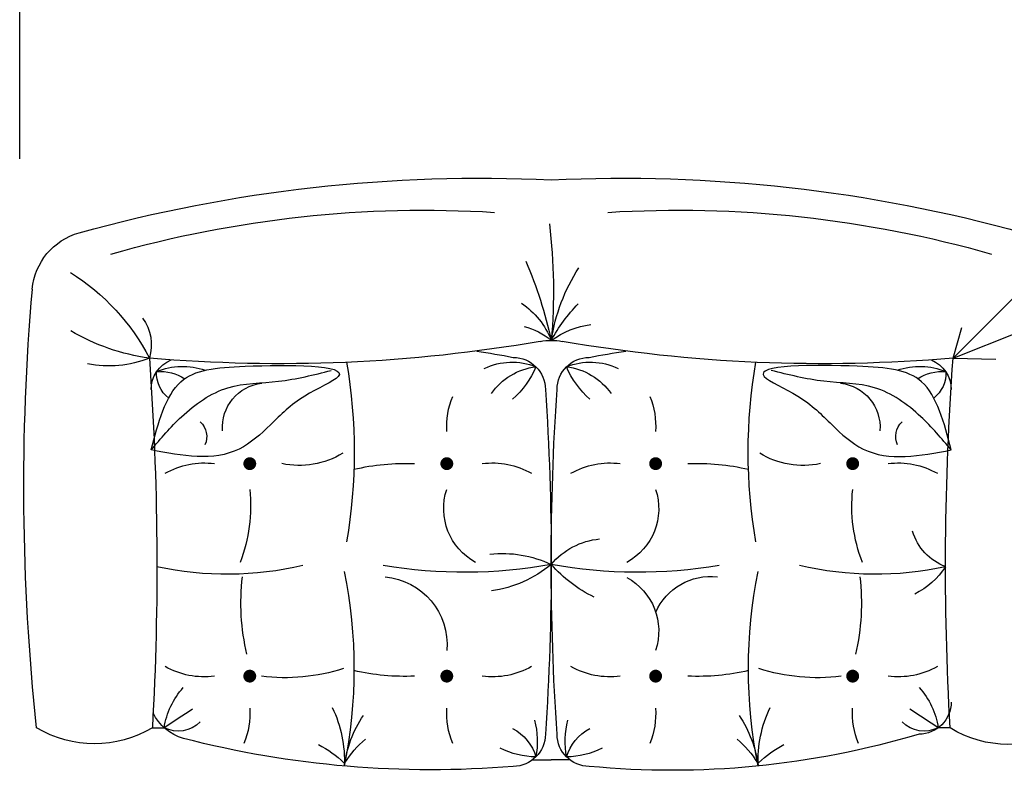
# Model space of a CAD drawing. Units: inches. Extents: x 3592 to 4861, y 1650 to 2243.
# Tile 9 of 30: x 4173 to 4219, y 1968 to 2003. Entities that reach past the tile are written whole.
import ezdxf

# ---------------------------------------------------------------- set-up
doc = ezdxf.new("R2010")
doc.units = ezdxf.units.IN
doc.layers.add('A-ANNO-DIMS', color=2, linetype='Continuous', lineweight=13)
doc.layers.add('A-FURN', color=9, linetype='Continuous', lineweight=13)
doc.layers.add('RA-AP-01$0$FURN', color=3, linetype='Continuous')
doc.styles.get("Standard").update_dxf_attribs({"font": 'arial.ttf'})
doc.dimstyles.new('ISO-25', dxfattribs={"dimtxt": 9, "dimasz": 2.5, "dimexe": 1.25, "dimexo": 0.625, "dimtad": 1, "dimlunit": 3, "dimtxsty": 'Standard', "dimcen": 2.5, "dimadec": 0, "dimazin": 0, "dimtfac": 1, "dimtmove": 0, "dimatfit": 3, "dimfxl": 1, "dimarcsym": 0})

# ---------------------------------------------------------------- blocks, each defined once
blk = doc.blocks.new('A$C6E322C05')
at = {"layer": 'RA-AP-01$0$FURN'}
for p, q in [((6.3919, -6.482), (6.5167, -6.3573)), ((6.3919, -6.482), (6.4334, -6.3775)), ((6.3919, -6.482), (6.3904, -6.4155)), ((6.3919, -6.482), (6.4393, -6.4682)), ((5.8172, -6.4867), (5.8172, -6.5051)), ((5.7672, -7.0775), (5.7672, -7.1067)), ((5.7672, -7.1359), (5.7672, -7.1067)), ((5.8172, -7.7267), (5.8172, -7.7084))]:
    blk.add_line(p, q, dxfattribs=at)
at = {"layer": 'RA-AP-01$0$FURN', "const_width": 0.01}
for points in [[(5.9025, -6.6381, 1), (5.8925, -6.6381, 1)], [(6.2228, -6.6381, -1), (6.2328, -6.6381, -1)], [(5.9025, -6.9444, -1), (5.8925, -6.9444, -1)], [(6.2228, -6.9444, 1), (6.2328, -6.9444, 1)], [(5.9025, -7.269, 1), (5.8925, -7.269, 1)], [(6.2228, -7.269, -1), (6.2328, -7.269, -1)], [(5.9025, -7.5753, -1), (5.8925, -7.5753, -1)], [(6.2228, -7.5753, 1), (6.2328, -7.5753, 1)]]:
    blk.add_lwpolyline(points, format="xyb", close=True, dxfattribs=at)
at = {"layer": 'RA-AP-01$0$FURN'}
for centre, radius, start, end in [((6.1922, -9.8397), 3.5528, 85.0473, 96.0589), ((6.4903, -6.3998), 0.1, 15.4995, 85.0473), ((5.9622, -6.3967), 0.1707, 148.1726, 211.8274), ((4.3367, -6.997), 2.3349, 357.3064, 15.4995), ((4.8466, -6.9097), 1.7752, 356.478, 15.9335), ((5.8573, -6.535), 0.05, 90, 180), ((6.0683, -2.0198), 4.4739, 266.7829, 274.1477), ((6.343, -6.535), 0.05, 22.5827, 90), ((8.747, -6.6855), 2.3639, 175.063, 189.8434), ((6.134, -6.5955), 0.1215, 123.1053, 153.7006), ((6.5659, -6.6031), 0.5101, 167.6182, 193.3122), ((6.1475, -6.4635), 0.0853, 200.7831, 253.0462), ((6.3679, -6.5411), 0.0479, 86.5753, 142.6834), ((6.3027, -6.4996), 0.0683, 326.673, 5.2184), ((6.2748, -6.5339), 0.1042, 340.4828, 22.8693), ((5.86, -6.527), 0.0479, 152.8071, 225.4025), ((5.7982, -6.6254), 0.1219, 48.0376, 81.0462), ((4.9043, -7.1366), 1.1102, 31.9329, 34.6665), ((6.0178, -6.5669), 0.1214, 150.1419, 187.6917), ((6.1075, -6.5669), 0.1214, 352.3083, 29.8581), ((7.0946, -6.9193), 1.3435, 163.3777, 185.4807), ((6.2698, -6.5402), 0.031, 245.776, 317.3789), ((6.2843, -6.6645), 0.0689, 6.4195, 94.4616), ((6.0116, -6.9762), 0.3517, 83.4125, 103.1675), ((6.1623, -6.3952), 0.2442, 248.9017, 275.9924), ((5.8396, -6.5171), 0.1213, 247.3376, 273.7315), ((6.1975, -6.6925), 0.3024, 173.0945, 197.5881), ((6.3545, -6.7151), 0.1295, 167.9901, 211.3796), ((5.6503, -6.6735), 0.1579, 315.4052, 333.0845), ((5.7659, -6.5936), 0.1916, 267.5853, 295.5831), ((5.9088, -6.0346), 0.7655, 258.6273, 281.4174), ((5.7331, -6.9697), 0.1864, 56.2926, 82.3818), ((5.6794, -6.9201), 0.1579, 40.3865, 58.0658), ((6.2459, -5.9772), 0.8233, 260.2449, 279.7551), ((6.2458, -6.8794), 0.3487, 166.8392, 182.4658), ((5.8795, -6.8794), 0.3487, 357.5342, 13.1608), ((5.9595, -6.8591), 0.093, 293.6025, 6.6107), ((6.8074, -6.9716), 0.7485, 170.3094, 190.3986), ((5.8396, -7.0655), 0.1213, 86.2685, 112.6624), ((5.9673, -7.035), 0.0954, 28.8034, 108.2253), ((6.158, -7.035), 0.0954, 71.7747, 151.1966), ((6.2857, -7.0655), 0.1213, 67.3376, 93.7315), ((5.087, -6.7913), 1.3309, 348.8964, 351.3771), ((6.0178, -7.0157), 0.1214, 172.3083, 209.8581), ((6.1075, -7.0157), 0.1214, 330.1419, 7.6917), ((6.2863, -7.0456), 0.0993, 337.9047, 25.6344), ((6.28, -7.0949), 0.0991, 6.9226, 55.1088), ((5.9042, -7.0857), 0.1324, 153.8888, 178.8007), ((6.2111, -6.9471), 0.2123, 205.9704, 228.742), ((5.9995, -7.0211), 0.1117, 309.9426, 354.6906), ((5.8073, -7.0476), 0.05, 180, 270), ((5.7515, -7.0133), 0.0726, 286.3559, 332.6775), ((6.4323, -6.9553), 0.1386, 221.2289, 247.0868), ((6.343, -7.0476), 0.05, 270, 360), ((6.3046, -7.0248), 0.1411, 324.485, 351.7973), ((6.3746, -6.8181), 0.292, 278.8152, 302.6921), ((6.2856, -6.8652), 0.2761, 298.9826, 313.6694), ((5.7956, -6.9527), 0.1324, 259.6959, 284.6078), ((6.0752, -3.1637), 3.943, 266.1043, 273.8957), ((6.3194, -7.1067), 0.1, 350.1566, 9.8434), ((5.8073, -7.1658), 0.05, 90, 180), ((6.0752, -11.0497), 3.943, 86.1043, 93.8957), ((6.2139, -7.2252), 0.1855, 140.3168, 172.0523), ((6.8074, -7.2418), 0.7485, 169.6011, 189.6906), ((5.9113, -7.1825), 0.1769, 353.6796, 25.3608), ((6.343, -7.1658), 0.05, 0, 90), ((6.4964, -7.9619), 0.8587, 83.0376, 95.1445), ((6.3757, -7.2207), 0.122, 33.7136, 69.041), ((6.3383, -7.1753), 0.1062, 14.3648, 40.2303), ((6.2695, -7.7891), 0.6986, 67.0091, 77.612), ((4.3367, -7.2164), 2.3349, 344.5005, 2.6936), ((5.7956, -7.2607), 0.1324, 75.3922, 100.3041), ((5.9042, -7.1277), 0.1324, 181.1993, 206.1112), ((5.7515, -7.2001), 0.0726, 27.3225, 73.6441), ((6.4323, -7.2581), 0.1386, 112.9132, 138.7711), ((6.28, -7.1185), 0.0991, 304.8912, 353.0774), ((6.2863, -7.1678), 0.0993, 334.3656, 22.0953), ((8.747, -7.5279), 2.3639, 170.1566, 184.937), ((6.0178, -7.1977), 0.1214, 150.1419, 187.6917), ((6.1075, -7.1977), 0.1214, 352.3083, 29.8581), ((7.291, -7.294), 1.5391, 175.2234, 194.4661), ((5.087, -7.4221), 1.3309, 8.6229, 11.1036), ((4.8466, -7.3037), 1.7752, 344.0665, 3.522), ((6.158, -7.1784), 0.0954, 208.8034, 288.2253), ((5.8396, -7.1479), 0.1213, 247.3376, 273.7315), ((5.9463, -7.3746), 0.106, 5.1859, 94.8073), ((6.2857, -7.1479), 0.1213, 266.2685, 292.6624), ((6.2458, -7.334), 0.3487, 177.5342, 193.1608), ((5.8795, -7.334), 0.3487, 346.8392, 2.4658), ((5.7331, -7.2437), 0.1864, 277.6182, 303.7074), ((5.6794, -7.2933), 0.1579, 301.9342, 319.6135), ((5.9088, -8.1788), 0.7655, 78.5826, 101.3727), ((6.2459, -8.2362), 0.8233, 80.2449, 99.7551), ((5.7659, -7.6198), 0.1916, 64.4169, 92.4147), ((5.6503, -7.5399), 0.1579, 26.9155, 44.5948), ((6.1975, -7.5209), 0.3024, 162.4119, 186.9055), ((6.3545, -7.4983), 0.1295, 148.6204, 192.0099), ((6.5659, -7.6103), 0.5101, 166.6878, 192.3818), ((6.2843, -7.5489), 0.0689, 265.5384, 353.5805), ((5.8396, -7.6963), 0.1213, 86.2685, 112.6624), ((6.1623, -7.8182), 0.2442, 84.0076, 111.0983), ((6.0116, -7.2373), 0.3517, 256.8325, 276.5875), ((6.0178, -7.6465), 0.1214, 172.3083, 209.8581), ((6.1075, -7.6465), 0.1214, 330.1419, 7.6917), ((5.86, -7.6864), 0.0479, 134.5975, 207.1929), ((6.2698, -7.6732), 0.031, 42.6211, 114.224), ((6.2748, -7.6795), 0.1042, 337.1307, 19.5172), ((4.9043, -7.0769), 1.1102, 325.3335, 328.0671), ((5.8732, -7.6577), 0.0754, 196.0166, 244.1254), ((5.7982, -7.588), 0.1219, 278.9538, 311.9624), ((6.3027, -7.7138), 0.0683, 354.7816, 33.327), ((6.343, -7.6785), 0.05, 270, 337.4173), ((6.3679, -7.6723), 0.0479, 217.3166, 273.4247), ((5.9667, -7.8167), 0.1745, 148.9518, 211.0482), ((6.0683, -12.1936), 4.4739, 85.8523, 93.2171), ((6.4123, -7.7988), 0.0705, 53.5874, 106.8661), ((6.5496, -7.7946), 0.1699, 158.1488, 191.1222), ((6.7131, -7.688), 0.3242, 187.6974, 210.7014), ((6.2371, -8.0321), 0.3382, 31.7436, 62.7697), ((6.4903, -7.8137), 0.1, 274.9527, 344.5005), ((6.1922, -4.3737), 3.5528, 263.9411, 274.9527)]:
    blk.add_arc(centre, radius, start, end, dxfattribs=at)
for points, knots in [([(6.2491, -6.4849), (6.2399, -6.5334), (6.2266, -6.6036), (6.2907, -6.674), (6.3321, -6.7134), (6.3818, -6.8312), (6.3817, -6.6297), (6.3708, -6.5166), (6.2912, -6.4959), (6.2491, -6.4849)], [0, 0, 0, 0, 0.1367587, 0.1981302, 0.267773, 0.3281195, 0.4737578, 0.5765194, 0.6920332, 0.6920332, 0.6920332, 0.6920332]), ([(6.2491, -6.4849), (6.2669, -6.4999), (6.3062, -6.533), (6.3538, -6.6001), (6.3525, -6.6851), (6.3659, -6.7377), (6.3727, -6.7646)], [0, 0, 0, 0, 0.0700185, 0.155078, 0.2344492, 0.3178049, 0.3178049, 0.3178049, 0.3178049]), ([(6.2491, -7.7285), (6.2399, -7.6801), (6.2266, -7.6099), (6.2907, -7.5394), (6.3321, -7.5001), (6.3818, -7.3822), (6.3817, -7.5838), (6.3708, -7.6968), (6.2912, -7.7175), (6.2491, -7.7285)], [0, 0, 0, 0, 0.1367587, 0.1981302, 0.267773, 0.3281195, 0.4737578, 0.5765194, 0.6920332, 0.6920332, 0.6920332, 0.6920332]), ([(6.2491, -7.7285), (6.2669, -7.7136), (6.3062, -7.6804), (6.3538, -7.6133), (6.3525, -7.5283), (6.3659, -7.4757), (6.3727, -7.4488)], [0, 0, 0, 0, 0.0700185, 0.155078, 0.2344492, 0.3178049, 0.3178049, 0.3178049, 0.3178049])]:
    blk.add_open_spline(points, degree=3, knots=knots, dxfattribs=at)
blk = doc.blocks.new('A$C44E37296')
at = {"layer": 'RA-AP-01$0$FURN', "xscale": -1}
blk.add_blockref('A$C6E322C05', (4.6545, 7.7124), dxfattribs=at)
blk = doc.blocks.new('*D165')
at = {"layer": 'A-ANNO-DIMS', "color": 0, "lineweight": -2, "transparency": 16777216}
for p, q in [((4173.347, 1996.551), (4173.347, 2015.717)), ((4247.079, 1996.551), (4247.079, 2015.717)), ((4175.847, 2014.467), (4244.579, 2014.467))]:
    blk.add_line(p, q, dxfattribs=at)
at = {"layer": 'A-ANNO-DIMS', "color": 0, "transparency": 16777216}
for points in [[(4175.847, 2014.884), (4175.847, 2014.051), (4173.347, 2014.467)], [(4244.579, 2014.884), (4244.579, 2014.051), (4247.079, 2014.467)]]:
    blk.add_solid(points, dxfattribs=at)
at = {"layer": 'Defpoints', "color": 0, "transparency": 16777216}
for p in [(4247.079, 2014.467), (4173.347, 1995.926), (4247.079, 1995.926)]:
    blk.add_point(p, dxfattribs=at)
at = {"layer": 'A-ANNO-DIMS', "color": 0, "transparency": 16777216, "insert": (4210.213, 2019.746), "char_height": 9, "attachment_point": 5}
blk.add_mtext('6\'-1 1/2"', dxfattribs=at)

msp = doc.modelspace()

# ---------------------------------------------------------------- block references
at = {"layer": 'A-FURN', "xscale": 29.98919001647196, "yscale": 29.98919001647196, "zscale": 29.98919001647196, "rotation": 270}
msp.add_blockref('A$C44E37296', (4179.961, 1935.164), dxfattribs=at)

# ---------------------------------------------------------------- dimensions: what is measured, and where the dimension line sits
at = {"layer": 'A-ANNO-DIMS'}
dim = msp.add_linear_dim(base=(4247.079, 2014.467), p1=(4173.347, 1995.926), p2=(4247.079, 1995.926), dimstyle='ISO-25', override={"dimdec": 1, "dimlfac": 1, "dimrnd": 0, "dimzin": 1, "dimdsep": 46, "dimlunit": 4, "dimfrac": 2}, dxfattribs=at)
dim.commit()
dim.dimension.update_dxf_attribs({"geometry": '*D165', "text_midpoint": (4210.213, 2019.746)})

doc.saveas('drawing.dxf')
